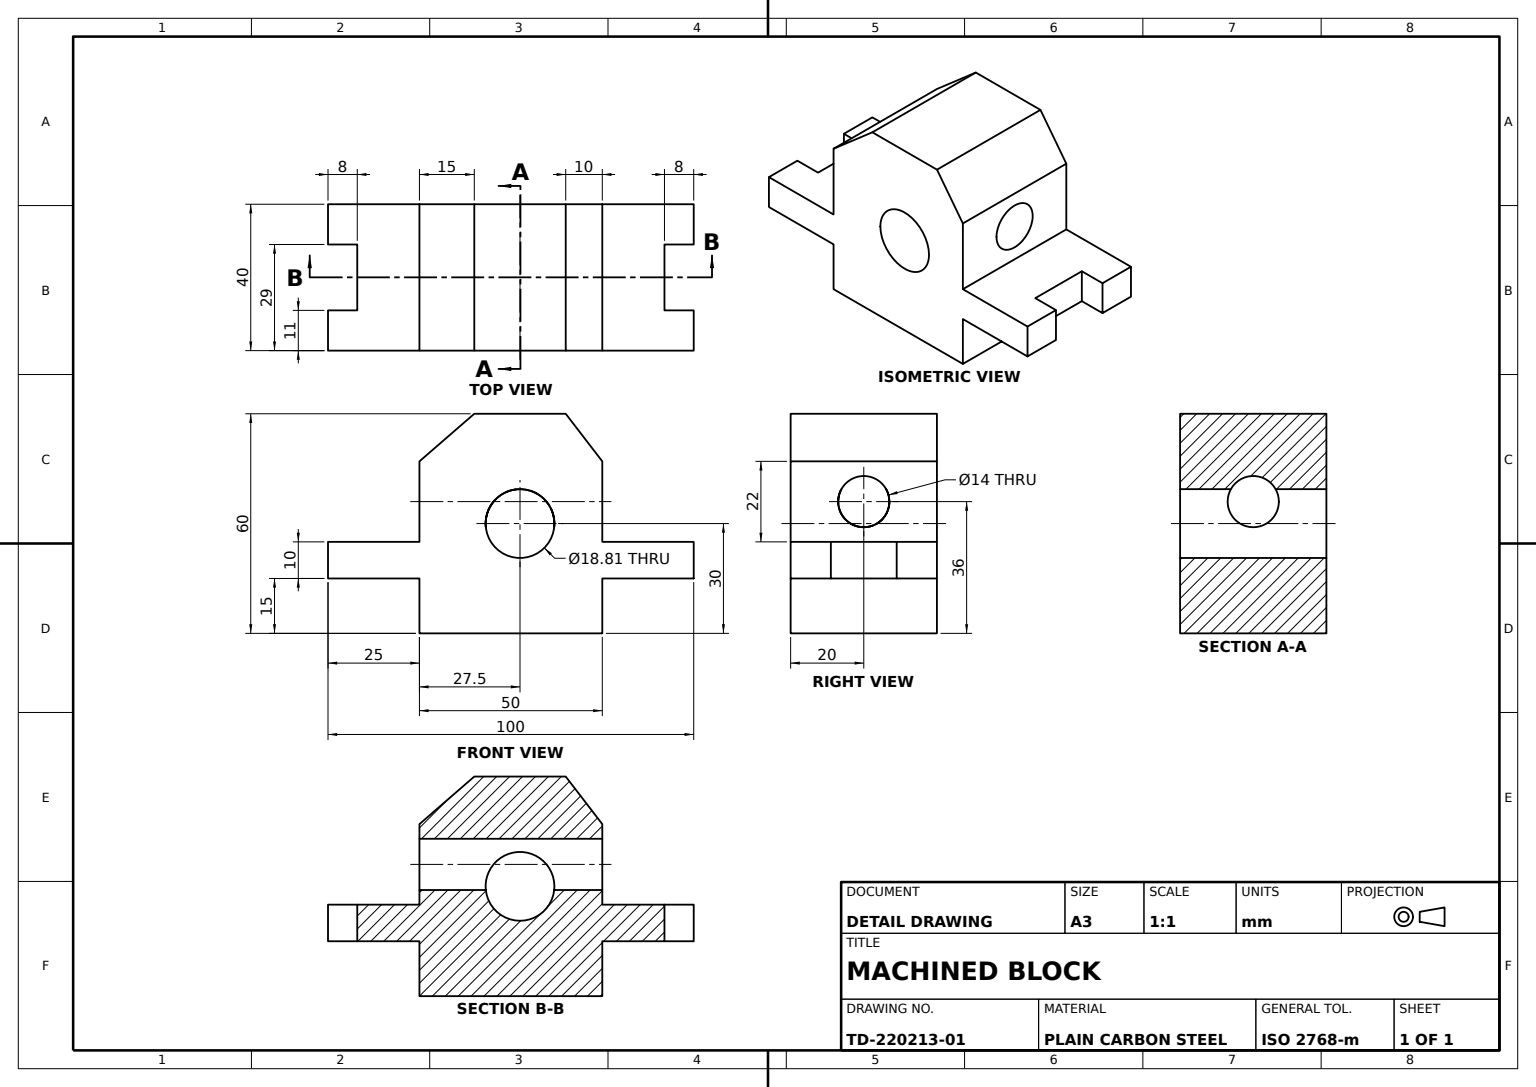
SolidWorks part; units mm, degrees
material "Plain Carbon Steel"
ref_plane "Front Plane" through (0, 0, 0) normal (0, 0, 1) x (1, 0, 0)
ref_plane "Top Plane" through (0, 0, 0) normal (0, 1, 0) x (1, 0, 0)
ref_plane "Right Plane" through (0, 0, 0) normal (1, 0, 0) x (0, 0, -1)
sketch "Bracket Profile Sketch" plane through (0, 0, 0) normal (0, 0, 1) x (1, 0, 0)
  line L0 (0, 0) -> (50, 0)
  line L1 (50, 0) -> (50, 15)
  line L2 (50, 15) -> (75, 15)
  line L3 (75, 15) -> (75, 25)
  line L4 (75, 25) -> (50, 25)
  line L5 (50, 25) -> (50, 47)
  line L6 (0, 0) -> (0, 15)
  line L7 (0, 15) -> (-25, 15)
  line L8 (-25, 15) -> (-25, 25)
  line L9 (-25, 25) -> (0, 25)
  line L10 (0, 25) -> (0, 47)
  line L14 (0, 47) -> (15, 60)
  line L15 (40, 60) -> (50, 47)
  line L16 (15, 60) -> (40, 60)
  dimension "D2" = 10
  dimension "D3" = 13
  dimension "D4" = 15
  dimension "D5" = 10
  dimension "D6" = 22
  dimension "D7" = 100
  dimension "D8" = 50
  dimension "D9" = 50
  dimension "D10" = 60
  dimension "D11" = 25
  dimension "D12" = 25
  dimension "D13" = 40
  dimension "D14" = 50
extrude "Bracket Body" add sketch "Bracket Profile Sketch" along normal blind 40 contours L0 L1 L2 L3 L4 L5 L15 L16 L14 L10 L9 L8 L7 L6
sketch "Front Bore Sketch" plane through (0, 0, 40) normal (0, 0, 1) x (1, 0, 0)
  line L0 (0, 0) -> (0, 15) construction
  line L1 (0, 0) -> (50, 0) construction
  circle A0 centre (27.5, 30) radius 9.4038
  dimension "D1" = 18.8075
  dimension "D2" = 27.5
  dimension "D3" = 30
extrude "Front Bore" cut sketch "Front Bore Sketch" against normal through all
sketch "Flange Notch Sketch" plane through (0, 25, 0) normal (0, 1, 0) x (1, 0, 0)
  line L0 (75, -11) -> (67, -11)
  line L1 (75, -40) -> (75, 0) construction
  line L2 (75, -11) -> (67, -11) construction
  line L3 (67, -11) -> (67, -29) construction
  line L4 (67, -29) -> (75, -29) construction
  line L5 (75, -29) -> (75, -11) construction
  line L6 (67, -11) -> (67, -29)
  line L7 (67, -29) -> (75, -29)
  line L8 (75, -29) -> (75, -11)
  line L9 (50, -40) -> (50, 0) construction
  line L10 (75, 0) -> (50, 0) construction
  dimension "D1" = 17
  dimension "D2" = 11
  dimension "D3" = 29
extrude "Flange Notch Cuts" cut sketch "Flange Notch Sketch" against normal blind 40
sketch "Flange Slot Sketch" plane through (0, 25, 0) normal (0, 1, 0) x (1, 0, 0)
  line L1 (-25, -40) -> (-25, 0) construction
  line L2 (-25, -11) -> (-17, -11)
  line L3 (-17, -11) -> (-17, -29)
  line L4 (-17, -29) -> (-25, -29)
  line L5 (-25, -29) -> (-25, -11)
  dimension "D1" = 8
  dimension "D2" = 11
  dimension "D3" = 29
extrude "Flange Slot Cut" cut sketch "Flange Slot Sketch" against normal blind 40
sketch "Cross Hole Sketch" plane through (50, 0, 0) normal (1, 0, 0) x (0, 0, -1)
  line L0 (0, 25) -> (0, 47) construction
  line L1 (-40, 47) -> (0, 47) construction
  circle A0 centre (-20, 36) radius 7
  dimension "D1" = 14
  dimension "D2" = 20
  dimension "D3" = 11
extrude "Cross Hole Ø14" cut sketch "Cross Hole Sketch" against normal through all
